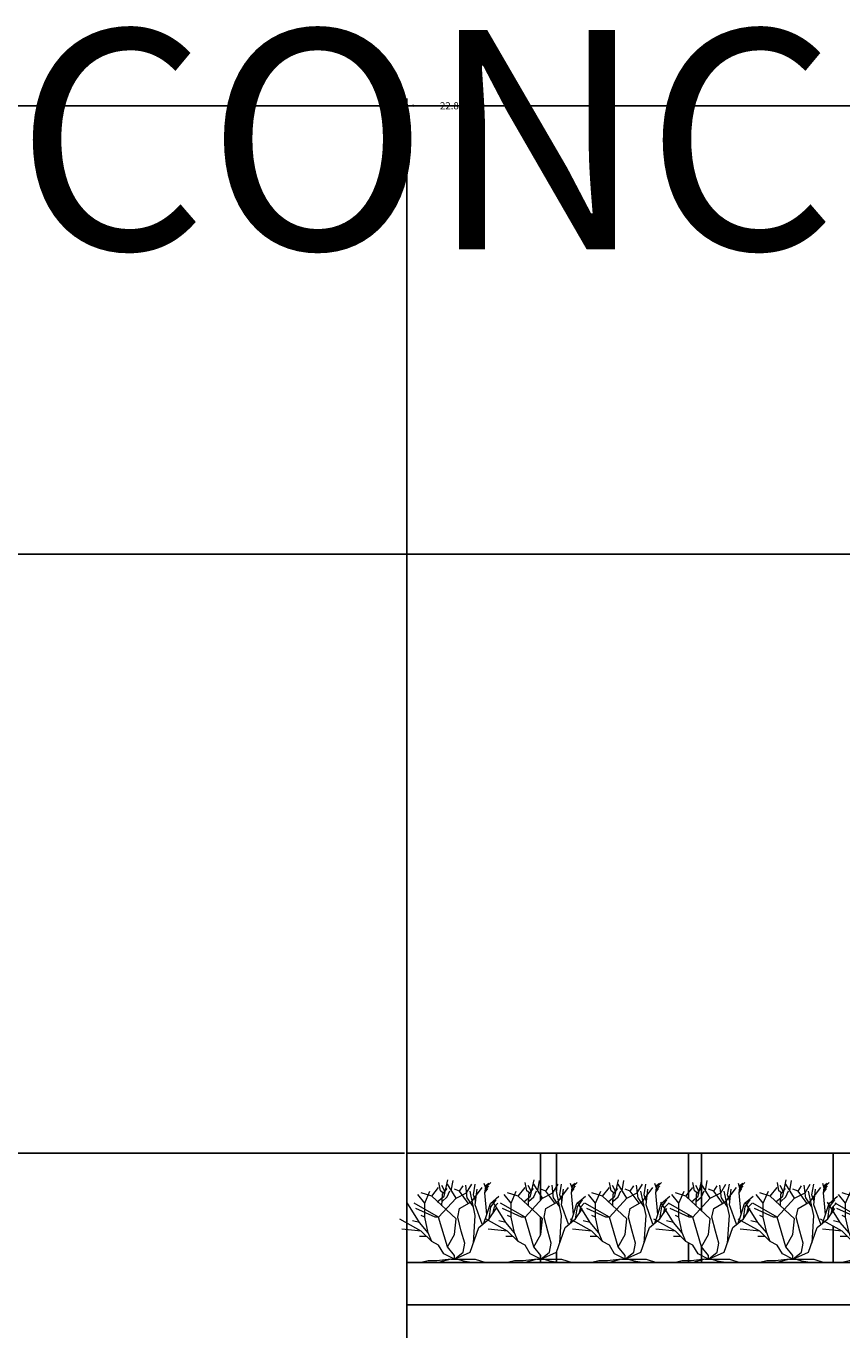
# Model space of a CAD drawing. Units: inches. Extents: x -117 to 121, y -77 to 40.
# Tile 15 of 45: x -85 to -65, y 7 to 40. Entities that reach past the tile are written whole.
import ezdxf

# ---------------------------------------------------------------- set-up
doc = ezdxf.new("R2010")
doc.units = ezdxf.units.IN
doc.header["$MEASUREMENT"] = 0
for name, color, linetype, lineweight in [('A-ANNO-DIMS', 2, 'Continuous', 18), ('A-ANNO-TEXT', 7, 'Continuous', 25), ('A-ELEV', 7, 'Continuous', 25), ('L-PLNT', 3, 'Continuous', 13)]:
    doc.layers.add(name, color=color, linetype=linetype, lineweight=lineweight)
doc.styles.get("Standard").update_dxf_attribs({"font": 'arial.ttf'})
doc.dimstyles.get("Standard").update_dxf_attribs({"dimtxt": 0.18, "dimasz": 0.18, "dimexe": 0.18, "dimexo": 0.0625, "dimgap": 0.09, "dimtad": 0, "dimtih": 1, "dimtoh": 1, "dimdec": 4, "dimzin": 0, "dimdsep": 46, "dimtxsty": 'Standard', "dimcen": 0.09, "dimadec": 0, "dimazin": 0, "dimtfac": 1, "dimtdec": 4, "dimtofl": 0, "dimtmove": 0, "dimatfit": 3, "dimfxl": 1, "dimtolj": 1, "dimtzin": 0, "dimarcsym": 0})

# ---------------------------------------------------------------- blocks, each defined once
blk = doc.blocks.new('*U3')
for p, q in [((-12.471, 19.775), (-12.898, 22.044)), ((-11.433, 18.289), (-10.457, 22.749)), ((-8.16, 17.76), (-10.56, 21.6)), ((-9.48, 19.775), (-8.992, 22.592)), ((-5.28, 19.2), (-3.84, 21.6)), ((-3.377, 18.602), (-2.888, 21.575)), ((-0.508, 21.888), (-0.081, 20.558)), ((0.041, 20.714), (1.384, 22.044)), ((0.102, 21.34), (0.835, 21.888)), ((-16.8, 16.32), (-18.72, 18.72)), ((-14.88, 18.24), (-17.76, 19.2)), ((-16.8, 16.32), (-15.36, 19.68)), ((-14.88, 18.24), (-12.96, 20.64)), ((-8.16, 12), (-14.88, 18.24)), ((-13.325, 16.724), (-11.433, 18.289)), ((-11.677, 19.071), (-12.471, 19.775)), ((-11.28, 19.619), (-12.104, 21.184)), ((-12.043, 15.628), (-11.921, 18.836)), ((-11.982, 16.802), (-10.579, 18.054)), ((-11.921, 18.836), (-10.64, 20.401)), ((-10.579, 18.054), (-9.846, 19.697)), ((-7.2, 19.68), (-8.64, 20.16)), ((-8.16, 17.76), (-5.28, 19.2)), ((-7.2, 19.68), (-6.24, 21.12)), ((-4.8, 16.32), (-7.2, 19.68)), ((-5.086, 17.741), (-5.513, 21.34)), ((-2.88, 12.96), (-4.32, 19.68)), ((-3.84, 16.8), (-0.96, 20.64)), ((-2.766, 16.802), (-3.377, 18.602)), ((-2.88, 15.84), (-2.4, 20.16)), ((-0.203, 19.149), (0.102, 21.34)), ((0.346, 13.203), (-0.203, 19.149)), ((-0.142, 19.384), (0.59, 20.401)), ((-0.02, 20.01), (0.896, 21.105)), ((1.323, 16.254), (3.642, 18.289)), ((-18.24, 11.04), (-21.755, 16.655)), ((-12.96, 12.48), (-19.68, 16.32)), ((-13.92, 12.48), (-19.2, 14.88)), ((-16.8, 12.48), (-16.8, 16.32)), ((-12.96, 12.48), (-8.16, 17.76)), ((-7.68, 12.48), (-7.2, 14.88)), ((-7.2, 14.88), (-3.84, 16.8)), ((-3.377, 15.315), (-5.086, 17.819)), ((-0.96, 10.56), (-2.88, 15.84)), ((0.346, 13.203), (1.323, 16.254)), ((0.96, 12), (1.44, 15.36)), ((0.96, 12), (2.88, 14.88)), ((1.44, 15.36), (2.88, 17.28)), ((1.92, 13.44), (2.4, 15.36)), ((2.4, 15.36), (3.36, 16.32)), ((-17.76, 8.64), (-23.663, 11.961)), ((-18.24, 11.04), (-20.16, 11.52)), ((-15.84, 8.16), (-18.24, 11.04)), ((-16.8, 12.48), (-17.76, 12.96)), ((-15.84, 8.16), (-16.8, 12.48)), ((-12.96, 12.48), (-13.92, 12.48)), ((-10.56, 4.32), (-12.96, 12.48)), ((-8.64, 7.68), (-8.16, 12)), ((-6.72, 8.64), (-7.68, 12.48)), ((-3.36, 5.28), (-2.88, 12.96)), ((-1.92, 9.6), (0.96, 12)), ((-0.48, 10.8), (0.346, 13.203)), ((-17.76, 8.64), (-23.128, 9.222)), ((-16.32, 7.2), (-18.24, 7.2)), ((-14.88, 5.76), (-17.76, 8.64)), ((-14.88, 5.76), (-15.84, 8.16)), ((-10.56, 4.32), (-8.64, 7.68)), ((-5.76, 5.28), (-6.72, 8.64)), ((-4.32, 2.88), (-1.92, 9.6)), ((-12.96, 4.8), (-14.88, 5.76)), ((-11.52, 2.4), (-12.96, 4.8)), ((-8.64, 1.92), (-10.56, 4.32)), ((-6.24, 2.88), (-5.76, 5.28)), ((-15.84, 0.48), (-17.76, 0)), ((-13.44, 0.48), (-15.84, 0.48)), ((-9.6, 0.96), (-13.44, 0.48)), ((-9.6, 0.96), (-12.96, 0)), ((-8.64, 0.96), (-11.52, 2.4)), ((-9.6, 0.96), (-7.68, 0.96)), ((-8.64, 0.96), (-4.32, 2.88)), ((-8.64, 0.96), (-6.24, 2.88)), ((-8.64, 0.96), (-8.64, 1.92)), ((-8.64, 0.96), (-2.88, 0.96)), ((-7.68, 0.96), (-6.24, 0.48)), ((-6.24, 0.48), (-3.36, 0)), ((-2.88, 0.96), (0, 0))]:
    blk.add_line(p, q)
blk = doc.blocks.new('*D9')
at = {"layer": 'A-ANNO-DIMS', "color": 0, "lineweight": -2, "transparency": 16777216}
for p, q in [((-75.804, 8.087), (-75.804, 38.61)), ((-75.624, 38.43), (-50.227, 38.43)), ((-24.044, 38.43), (-49.44, 38.43)), ((-23.864, 8.087), (-23.864, 38.61))]:
    blk.add_line(p, q, dxfattribs=at)
at = {"layer": 'A-ANNO-DIMS', "color": 0, "transparency": 16777216}
for points in [[(-75.624, 38.46), (-75.624, 38.4), (-75.804, 38.43)], [(-24.044, 38.46), (-24.044, 38.4), (-23.864, 38.43)]]:
    blk.add_solid(points, dxfattribs=at)
at = {"layer": 'Defpoints', "color": 0, "transparency": 16777216}
for p in [(-23.864, 38.43), (-75.804, 8.025), (-23.864, 8.025)]:
    blk.add_point(p, dxfattribs=at)
at = {"layer": 'A-ANNO-DIMS', "color": 0, "transparency": 16777216, "insert": (-49.834, 38.43), "char_height": 0.18, "attachment_point": 5}
blk.add_mtext('\\A1;51.94', dxfattribs=at)
blk = doc.blocks.new('*D13')
at = {"layer": 'A-ANNO-DIMS', "color": 0, "lineweight": -2, "transparency": 16777216}
for p, q in [((-2.663, 27.063), (-117.024, 27.063)), ((-116.844, 26.883), (-116.844, -16.974)), ((-116.844, -61.196), (-116.844, -17.338)), ((-106.096, -61.376), (-117.024, -61.376))]:
    blk.add_line(p, q, dxfattribs=at)
at = {"layer": 'A-ANNO-DIMS', "color": 0, "transparency": 16777216}
for points in [[(-116.874, 26.883), (-116.814, 26.883), (-116.844, 27.063)], [(-116.874, -61.196), (-116.814, -61.196), (-116.844, -61.376)]]:
    blk.add_solid(points, dxfattribs=at)
at = {"layer": 'Defpoints', "color": 0, "transparency": 16777216}
for p in [(-2.6, 27.063), (-116.844, -61.376), (-106.034, -61.376)]:
    blk.add_point(p, dxfattribs=at)
at = {"layer": 'A-ANNO-DIMS', "color": 0, "transparency": 16777216, "insert": (-116.844, -17.156), "char_height": 0.18, "attachment_point": 5}
blk.add_mtext('\\A1;88.44', dxfattribs=at)
blk = doc.blocks.new('*D20')
at = {"layer": 'A-ANNO-DIMS', "color": 0, "lineweight": -2, "transparency": 16777216}
for p, q in [((-75.866, 11.871), (-117.024, 11.871)), ((-116.844, 11.691), (-116.844, 0.051)), ((-116.844, -11.953), (-116.844, -0.313)), ((-94.498, -12.133), (-117.024, -12.133))]:
    blk.add_line(p, q, dxfattribs=at)
at = {"layer": 'A-ANNO-DIMS', "color": 0, "transparency": 16777216}
for points in [[(-116.874, 11.691), (-116.814, 11.691), (-116.844, 11.871)], [(-116.874, -11.953), (-116.814, -11.953), (-116.844, -12.133)]]:
    blk.add_solid(points, dxfattribs=at)
at = {"layer": 'Defpoints', "color": 0, "transparency": 16777216}
for p in [(-75.804, 11.871), (-116.844, -12.133), (-94.436, -12.133)]:
    blk.add_point(p, dxfattribs=at)
at = {"layer": 'A-ANNO-DIMS', "color": 0, "transparency": 16777216, "insert": (-116.844, -0.131), "char_height": 0.18, "attachment_point": 5}
blk.add_mtext('\\A1;24.004', dxfattribs=at)
blk = doc.blocks.new('*D21')
at = {"layer": 'A-ANNO-DIMS', "color": 0, "lineweight": -2, "transparency": 16777216}
for p, q in [((-106.034, -61.313), (-106.034, 38.61)), ((-105.854, 38.43), (-91.382, 38.43)), ((-75.984, 38.43), (-90.455, 38.43)), ((-75.804, 8.087), (-75.804, 38.61))]:
    blk.add_line(p, q, dxfattribs=at)
at = {"layer": 'A-ANNO-DIMS', "color": 0, "transparency": 16777216}
for points in [[(-105.854, 38.46), (-105.854, 38.4), (-106.034, 38.43)], [(-75.984, 38.46), (-75.984, 38.4), (-75.804, 38.43)]]:
    blk.add_solid(points, dxfattribs=at)
at = {"layer": 'Defpoints', "color": 0, "transparency": 16777216}
for p in [(-75.804, 38.43), (-75.804, 8.025), (-106.034, -61.376)]:
    blk.add_point(p, dxfattribs=at)
at = {"layer": 'A-ANNO-DIMS', "color": 0, "transparency": 16777216, "insert": (-90.919, 38.43), "char_height": 0.18, "attachment_point": 5}
blk.add_mtext('\\A1;30.230', dxfattribs=at)
blk = doc.blocks.new('*D40')
at = {"layer": 'A-ANNO-DIMS', "color": 0, "lineweight": -2, "transparency": 16777216}
for p, q in [((-86.023, -13.677), (-86.023, 38.61)), ((-85.843, 38.43), (-75.056, 38.43)), ((-63.339, 38.43), (-74.126, 38.43)), ((-63.159, -13.677), (-63.159, 38.61))]:
    blk.add_line(p, q, dxfattribs=at)
at = {"layer": 'A-ANNO-DIMS', "color": 0, "transparency": 16777216}
for points in [[(-85.843, 38.46), (-85.843, 38.4), (-86.023, 38.43)], [(-63.339, 38.46), (-63.339, 38.4), (-63.159, 38.43)]]:
    blk.add_solid(points, dxfattribs=at)
at = {"layer": 'Defpoints', "color": 0, "transparency": 16777216}
for p in [(-63.159, 38.43), (-86.023, -13.74), (-63.159, -13.74)]:
    blk.add_point(p, dxfattribs=at)
at = {"layer": 'A-ANNO-DIMS', "color": 0, "transparency": 16777216, "insert": (-74.591, 38.43), "char_height": 0.18, "attachment_point": 5}
blk.add_mtext('\\A1;22.864', dxfattribs=at)

msp = doc.modelspace()

# ---------------------------------------------------------------- linework, layer by layer
at = {"layer": 'A-ELEV'}
for p, q in [((-75.8037, 9.0994), (-75.8037, 11.8711)), ((-75.8037, 11.8711), (-23.8637, 11.8711)), ((-72.4168, 10.68), (-72.4168, 11.8711)), ((-72.0149, 10.9094), (-72.0149, 11.8711)), ((-68.6636, 10.7103), (-68.6636, 11.8711)), ((-68.3405, 10.4102), (-68.3405, 11.8711)), ((-65.0021, 10.6356), (-65.0021, 11.8711)), ((-72.0149, 10.6195), (-72.0149, 10.635)), ((-68.6636, 10.2543), (-68.6636, 10.3068)), ((-65.0021, 10.4066), (-65.0021, 10.5164)), ((-72.4168, 9.7979), (-72.4168, 10.2475)), ((-65.0021, 9.0994), (-65.0021, 10.0212)), ((-68.6636, 9.0994), (-68.6636, 9.5922)), ((-72.4168, 9.0994), (-72.4168, 9.2797)), ((-72.0149, 9.0994), (-72.0149, 9.3633)), ((-68.3405, 9.0994), (-68.3405, 9.5041)), ((-23.8637, 9.0994), (-75.8037, 9.0994)), ((-75.8037, 9.0994), (-75.8037, -3.0042)), ((-23.8637, 8.0246), (-75.8037, 8.0246))]:
    msp.add_line(p, q, dxfattribs=at)

# ---------------------------------------------------------------- block references
at = {"layer": 'L-PLNT', "xscale": 0.0920717077623056, "yscale": 0.0920717077623056, "zscale": 0.0920717077623056}
for p in [(-73.8066, 9.0979), (-71.6172, 9.0979), (-69.4788, 9.0979), (-67.3657, 9.0979), (-65.2273, 9.0979), (-63.1397, 9.0979)]:
    msp.add_blockref('*U3', p, dxfattribs=at)

# ---------------------------------------------------------------- texts
at = {"layer": 'A-ANNO-TEXT'}
msp.add_text('CONCEPTUAL    GOOD   VIBE   CAFE   DESIGN', height=5.56486, dxfattribs=at).set_placement((-85.726, 34.7863))

# ---------------------------------------------------------------- dimensions: what is measured, and where the dimension line sits
at = {"layer": 'A-ANNO-DIMS'}
for base, p1, p2, override, picture, middle in [((-75.8037, 38.4297), (-106.0338, -61.3756), (-75.8037, 8.0246), {"dimdec": 3, "dimlfac": 1, "dimrnd": 0, "dimzin": 0, "dimdsep": 46, "dimlunit": 2}, '*D21', (-90.9187, 38.4297)), ((-63.1589, 38.4297), (-86.0225, -13.74), (-63.1589, -13.74), {"dimdec": 3, "dimlfac": 1, "dimrnd": 0, "dimzin": 0, "dimdsep": 46, "dimlunit": 2}, '*D40', (-74.5907, 38.4297)), ((-23.8637, 38.4297), (-75.8037, 8.0246), (-23.8637, 8.0246), {"dimdec": 2, "dimlfac": 1, "dimrnd": 0, "dimzin": 0, "dimdsep": 46, "dimlunit": 2}, '*D9', (-49.8337, 38.4297))]:
    dim = msp.add_linear_dim(base=base, p1=p1, p2=p2, dimstyle='Standard', override=override, dxfattribs=at)
    dim.commit()
    dim.dimension.update_dxf_attribs({"geometry": picture, "text_midpoint": middle})
for base, p1, p2, override, picture, middle in [((-116.8438, -61.3756), (-2.6001, 27.0634), (-106.0338, -61.3756), {"dimdec": 2, "dimlfac": 1, "dimrnd": 0, "dimzin": 0, "dimdsep": 46, "dimlunit": 2}, '*D13', (-116.8438, -17.1561)), ((-116.84377, -12.13336), (-75.80372, 11.87111), (-94.43553, -12.13336), {"dimdec": 3, "dimlfac": 1, "dimrnd": 0, "dimzin": 0, "dimdsep": 46, "dimlunit": 2}, '*D20', (-116.84377, -0.13113))]:
    dim = msp.add_linear_dim(base=base, p1=p1, p2=p2, angle=90, dimstyle='Standard', override=override, dxfattribs=at)
    dim.commit()
    dim.dimension.update_dxf_attribs({"geometry": picture, "text_midpoint": middle})

doc.saveas('drawing.dxf')
